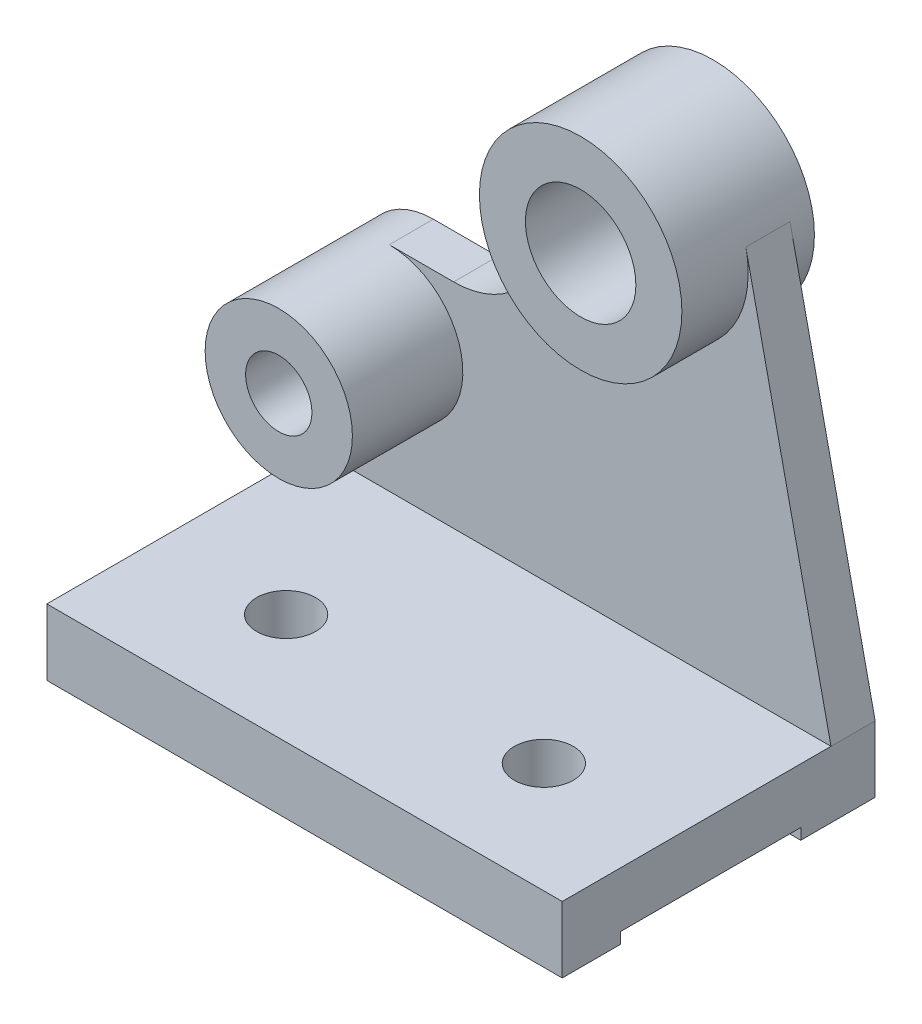
ISO-10303-21;
HEADER;
FILE_DESCRIPTION(('STEP AP214'),'2;1');
FILE_NAME('part.step','',(''),(''),'','','');
FILE_SCHEMA(('AUTOMOTIVE_DESIGN { 1 0 10303 214 1 1 1 1 }'));
ENDSEC;
DATA;
#1=APPLICATION_CONTEXT('core data for automotive mechanical design processes');
#2=APPLICATION_PROTOCOL_DEFINITION('international standard','automotive_design',2000,#1);
#3=PRODUCT_CONTEXT('',#1,'mechanical');
#4=PRODUCT('Part','Part','',(#3));
#5=PRODUCT_RELATED_PRODUCT_CATEGORY('part','',(#4));
#6=PRODUCT_DEFINITION_FORMATION('','',#4);
#7=PRODUCT_DEFINITION_CONTEXT('part definition',#1,'design');
#8=PRODUCT_DEFINITION('design','',#6,#7);
#9=PRODUCT_DEFINITION_SHAPE('','',#8);
#10=(LENGTH_UNIT() NAMED_UNIT(*) SI_UNIT(.MILLI.,.METRE.));
#11=(NAMED_UNIT(*) PLANE_ANGLE_UNIT() SI_UNIT($,.RADIAN.));
#12=(NAMED_UNIT(*) SI_UNIT($,.STERADIAN.) SOLID_ANGLE_UNIT());
#13=UNCERTAINTY_MEASURE_WITH_UNIT(LENGTH_MEASURE(1.E-05),#10,'distance_accuracy_value','');
#14=(GEOMETRIC_REPRESENTATION_CONTEXT(3) GLOBAL_UNCERTAINTY_ASSIGNED_CONTEXT((#13)) GLOBAL_UNIT_ASSIGNED_CONTEXT((#10,
#11,#12)) REPRESENTATION_CONTEXT('',''));
#15=CARTESIAN_POINT('',(0.,0.,0.));
#16=DIRECTION('',(0.,0.,1.));
#17=DIRECTION('',(1.,0.,0.));
#18=AXIS2_PLACEMENT_3D('',#15,#16,#17);
#19=CARTESIAN_POINT('',(-90.,-118.,85.));
#20=DIRECTION('',(0.,1.,0.));
#21=DIRECTION('',(0.,0.,1.));
#22=AXIS2_PLACEMENT_3D('',#19,#20,#21);
#23=PLANE('',#22);
#24=DIRECTION('',(0.,0.,-1.));
#25=VECTOR('',#24,1.);
#26=CARTESIAN_POINT('',(50.,-118.,85.));
#27=LINE('',#26,#25);
#28=CARTESIAN_POINT('',(50.0000000000001,-118.,20.2114764511151));
#29=VERTEX_POINT('',#28);
#30=CARTESIAN_POINT('',(50.,-118.,0.));
#31=VERTEX_POINT('',#30);
#32=EDGE_CURVE('E183',#29,#31,#27,.T.);
#33=ORIENTED_EDGE('',*,*,#32,.F.);
#34=DIRECTION('',(-1.,0.,0.));
#35=VECTOR('',#34,1.);
#36=CARTESIAN_POINT('',(50.0000000000001,-118.,20.2114764511151));
#37=LINE('',#36,#35);
#38=CARTESIAN_POINT('',(-90.,-118.,20.2114764511151));
#39=VERTEX_POINT('',#38);
#40=EDGE_CURVE('E240',#29,#39,#37,.T.);
#41=ORIENTED_EDGE('',*,*,#40,.T.);
#42=DIRECTION('',(0.,0.,-1.));
#43=VECTOR('',#42,1.);
#44=CARTESIAN_POINT('',(-90.,-118.,85.));
#45=LINE('',#44,#43);
#46=CARTESIAN_POINT('',(-90.,-118.,0.));
#47=VERTEX_POINT('',#46);
#48=EDGE_CURVE('E189',#39,#47,#45,.T.);
#49=ORIENTED_EDGE('',*,*,#48,.T.);
#50=DIRECTION('',(1.,0.,0.));
#51=VECTOR('',#50,1.);
#52=CARTESIAN_POINT('',(-90.,-118.,0.));
#53=LINE('',#52,#51);
#54=EDGE_CURVE('E279',#47,#31,#53,.T.);
#55=ORIENTED_EDGE('',*,*,#54,.T.);
#56=EDGE_LOOP('',(#33,#41,#49,#55));
#57=FACE_BOUND('',#56,.T.);
#58=ADVANCED_FACE('F41',(#57),#23,.F.);
#59=CARTESIAN_POINT('',(-70.,-62.,85.));
#60=DIRECTION('',(0.,0.,1.));
#61=DIRECTION('',(1.,0.,0.));
#62=AXIS2_PLACEMENT_3D('',#59,#60,#61);
#63=PLANE('',#62);
#64=DIRECTION('',(0.,1.,0.));
#65=VECTOR('',#64,1.);
#66=CARTESIAN_POINT('',(50.,-118.,85.));
#67=LINE('',#66,#65);
#68=CARTESIAN_POINT('',(50.,-118.,85.));
#69=VERTEX_POINT('',#68);
#70=CARTESIAN_POINT('',(50.,-100.,85.));
#71=VERTEX_POINT('',#70);
#72=EDGE_CURVE('E165',#69,#71,#67,.T.);
#73=ORIENTED_EDGE('',*,*,#72,.T.);
#74=DIRECTION('',(-1.,0.,0.));
#75=VECTOR('',#74,1.);
#76=CARTESIAN_POINT('',(50.,-100.,85.));
#77=LINE('',#76,#75);
#78=CARTESIAN_POINT('',(-90.,-100.,85.));
#79=VERTEX_POINT('',#78);
#80=EDGE_CURVE('E246',#71,#79,#77,.T.);
#81=ORIENTED_EDGE('',*,*,#80,.T.);
#82=DIRECTION('',(0.,-1.,0.));
#83=VECTOR('',#82,1.);
#84=CARTESIAN_POINT('',(-90.,-62.,85.));
#85=LINE('',#84,#83);
#86=CARTESIAN_POINT('',(-90.,-118.,85.));
#87=VERTEX_POINT('',#86);
#88=EDGE_CURVE('E272',#79,#87,#85,.T.);
#89=ORIENTED_EDGE('',*,*,#88,.T.);
#90=DIRECTION('',(1.,0.,0.));
#91=VECTOR('',#90,1.);
#92=CARTESIAN_POINT('',(-90.,-118.,85.));
#93=LINE('',#92,#91);
#94=EDGE_CURVE('E169',#87,#69,#93,.T.);
#95=ORIENTED_EDGE('',*,*,#94,.T.);
#96=EDGE_LOOP('',(#73,#81,#89,#95));
#97=FACE_BOUND('',#96,.T.);
#98=ADVANCED_FACE('F352',(#97),#63,.T.);
#99=CARTESIAN_POINT('',(-70.,-62.,85.));
#100=DIRECTION('',(0.,0.,-1.));
#101=DIRECTION('',(-1.,0.,0.));
#102=AXIS2_PLACEMENT_3D('',#99,#100,#101);
#103=CYLINDRICAL_SURFACE('',#102,20.);
#104=DIRECTION('',(0.,0.,-1.));
#105=VECTOR('',#104,1.);
#106=CARTESIAN_POINT('',(-90.,-62.,85.));
#107=LINE('',#106,#105);
#108=CARTESIAN_POINT('',(-90.,-62.,12.));
#109=VERTEX_POINT('',#108);
#110=CARTESIAN_POINT('',(-90.,-62.,0.));
#111=VERTEX_POINT('',#110);
#112=EDGE_CURVE('E151',#109,#111,#107,.T.);
#113=ORIENTED_EDGE('',*,*,#112,.F.);
#114=CARTESIAN_POINT('',(-70.,-62.,12.));
#115=DIRECTION('',(0.,0.,1.));
#116=DIRECTION('',(1.,0.,0.));
#117=AXIS2_PLACEMENT_3D('',#114,#115,#116);
#118=CIRCLE('',#117,20.);
#119=CARTESIAN_POINT('',(-70.,-42.,12.));
#120=VERTEX_POINT('',#119);
#121=EDGE_CURVE('E11',#120,#109,#118,.F.);
#122=ORIENTED_EDGE('',*,*,#121,.F.);
#123=DIRECTION('',(0.,0.,-1.));
#124=VECTOR('',#123,1.);
#125=CARTESIAN_POINT('',(-70.,-42.,85.));
#126=LINE('',#125,#124);
#127=CARTESIAN_POINT('',(-70.,-42.,0.));
#128=VERTEX_POINT('',#127);
#129=EDGE_CURVE('E146',#120,#128,#126,.T.);
#130=ORIENTED_EDGE('',*,*,#129,.T.);
#131=CARTESIAN_POINT('',(-70.,-62.,0.));
#132=DIRECTION('',(0.,0.,1.));
#133=DIRECTION('',(1.,0.,0.));
#134=AXIS2_PLACEMENT_3D('',#131,#132,#133);
#135=CIRCLE('',#134,20.);
#136=EDGE_CURVE('E269',#128,#111,#135,.T.);
#137=ORIENTED_EDGE('',*,*,#136,.T.);
#138=EDGE_LOOP('',(#113,#122,#130,#137));
#139=FACE_BOUND('',#138,.T.);
#140=CARTESIAN_POINT('',(-70.,-62.,42.));
#141=DIRECTION('',(0.,0.,1.));
#142=DIRECTION('',(1.,0.,0.));
#143=AXIS2_PLACEMENT_3D('',#140,#141,#142);
#144=CIRCLE('',#143,20.);
#145=CARTESIAN_POINT('',(-50.,-62.,42.));
#146=VERTEX_POINT('',#145);
#147=EDGE_CURVE('E208',#146,#146,#144,.T.);
#148=ORIENTED_EDGE('',*,*,#147,.F.);
#149=EDGE_LOOP('',(#148));
#150=FACE_BOUND('',#149,.T.);
#151=ADVANCED_FACE('F43',(#139,#150),#103,.T.);
#152=CARTESIAN_POINT('',(-90.,-62.,85.));
#153=DIRECTION('',(1.,0.,0.));
#154=DIRECTION('',(0.,1.,0.));
#155=AXIS2_PLACEMENT_3D('',#152,#153,#154);
#156=PLANE('',#155);
#157=ORIENTED_EDGE('',*,*,#48,.F.);
#158=DIRECTION('',(0.,-1.,0.));
#159=VECTOR('',#158,1.);
#160=CARTESIAN_POINT('',(-90.,-118.,20.2114764511151));
#161=LINE('',#160,#159);
#162=CARTESIAN_POINT('',(-90.,-115.,20.2114764511151));
#163=VERTEX_POINT('',#162);
#164=EDGE_CURVE('E226',#163,#39,#161,.T.);
#165=ORIENTED_EDGE('',*,*,#164,.F.);
#166=DIRECTION('',(0.,0.,-1.));
#167=VECTOR('',#166,1.);
#168=CARTESIAN_POINT('',(-90.,-115.,20.2114764511151));
#169=LINE('',#168,#167);
#170=CARTESIAN_POINT('',(-90.,-115.,69.2114764511151));
#171=VERTEX_POINT('',#170);
#172=EDGE_CURVE('E231',#171,#163,#169,.T.);
#173=ORIENTED_EDGE('',*,*,#172,.F.);
#174=DIRECTION('',(0.,1.,0.));
#175=VECTOR('',#174,1.);
#176=CARTESIAN_POINT('',(-90.,-118.,69.2114764511151));
#177=LINE('',#176,#175);
#178=CARTESIAN_POINT('',(-90.,-118.,69.2114764511151));
#179=VERTEX_POINT('',#178);
#180=EDGE_CURVE('E237',#179,#171,#177,.T.);
#181=ORIENTED_EDGE('',*,*,#180,.F.);
#182=EDGE_CURVE('E186',#87,#179,#45,.T.);
#183=ORIENTED_EDGE('',*,*,#182,.F.);
#184=ORIENTED_EDGE('',*,*,#88,.F.);
#185=DIRECTION('',(0.,0.,1.));
#186=VECTOR('',#185,1.);
#187=CARTESIAN_POINT('',(-90.,-100.,85.));
#188=LINE('',#187,#186);
#189=CARTESIAN_POINT('',(-90.,-100.,12.));
#190=VERTEX_POINT('',#189);
#191=EDGE_CURVE('E264',#190,#79,#188,.T.);
#192=ORIENTED_EDGE('',*,*,#191,.F.);
#193=DIRECTION('',(0.,-1.,0.));
#194=VECTOR('',#193,1.);
#195=CARTESIAN_POINT('',(-90.,-62.,12.));
#196=LINE('',#195,#194);
#197=EDGE_CURVE('E263',#109,#190,#196,.T.);
#198=ORIENTED_EDGE('',*,*,#197,.F.);
#199=ORIENTED_EDGE('',*,*,#112,.T.);
#200=DIRECTION('',(0.,-1.,0.));
#201=VECTOR('',#200,1.);
#202=CARTESIAN_POINT('',(-90.,-62.,0.));
#203=LINE('',#202,#201);
#204=EDGE_CURVE('E273',#111,#47,#203,.T.);
#205=ORIENTED_EDGE('',*,*,#204,.T.);
#206=EDGE_LOOP('',(#157,#165,#173,#181,#183,#184,#192,#198,#199,#205));
#207=FACE_BOUND('',#206,.T.);
#208=ADVANCED_FACE('F303',(#207),#156,.F.);
#209=CARTESIAN_POINT('',(50.,-100.,85.));
#210=DIRECTION('',(-0.97694867206773,-0.213474336033865,0.));
#211=DIRECTION('',(0.213474336033865,-0.97694867206773,0.));
#212=AXIS2_PLACEMENT_3D('',#209,#210,#211);
#213=PLANE('',#212);
#214=DIRECTION('',(-0.213474336033865,0.97694867206773,0.));
#215=VECTOR('',#214,1.);
#216=CARTESIAN_POINT('',(50.,-100.,12.));
#217=LINE('',#216,#215);
#218=CARTESIAN_POINT('',(50.,-100.,12.));
#219=VERTEX_POINT('',#218);
#220=CARTESIAN_POINT('',(26.8660884818626,5.87054424093129,12.));
#221=VERTEX_POINT('',#220);
#222=EDGE_CURVE('E258',#219,#221,#217,.T.);
#223=ORIENTED_EDGE('',*,*,#222,.F.);
#224=DIRECTION('',(0.,0.,-1.));
#225=VECTOR('',#224,1.);
#226=CARTESIAN_POINT('',(50.,-100.,85.));
#227=LINE('',#226,#225);
#228=CARTESIAN_POINT('',(50.,-100.,0.));
#229=VERTEX_POINT('',#228);
#230=EDGE_CURVE('E181',#219,#229,#227,.T.);
#231=ORIENTED_EDGE('',*,*,#230,.T.);
#232=DIRECTION('',(-0.213474336033865,0.97694867206773,0.));
#233=VECTOR('',#232,1.);
#234=CARTESIAN_POINT('',(50.,-100.,0.));
#235=LINE('',#234,#233);
#236=CARTESIAN_POINT('',(26.8660884818626,5.87054424093128,0.));
#237=VERTEX_POINT('',#236);
#238=EDGE_CURVE('E282',#229,#237,#235,.T.);
#239=ORIENTED_EDGE('',*,*,#238,.T.);
#240=DIRECTION('',(0.,0.,-1.));
#241=VECTOR('',#240,1.);
#242=CARTESIAN_POINT('',(26.8660884818626,5.87054424093128,85.));
#243=LINE('',#242,#241);
#244=EDGE_CURVE('E178',#221,#237,#243,.T.);
#245=ORIENTED_EDGE('',*,*,#244,.F.);
#246=EDGE_LOOP('',(#223,#231,#239,#245));
#247=FACE_BOUND('',#246,.T.);
#248=ADVANCED_FACE('F319',(#247),#213,.F.);
#249=CARTESIAN_POINT('',(0.,0.,85.));
#250=DIRECTION('',(0.,0.,-1.));
#251=DIRECTION('',(-1.,0.,0.));
#252=AXIS2_PLACEMENT_3D('',#249,#250,#251);
#253=CYLINDRICAL_SURFACE('',#252,27.5);
#254=DIRECTION('',(0.,0.,-1.));
#255=VECTOR('',#254,1.);
#256=CARTESIAN_POINT('',(-27.5,0.,85.));
#257=LINE('',#256,#255);
#258=CARTESIAN_POINT('',(-27.5,0.,12.));
#259=VERTEX_POINT('',#258);
#260=CARTESIAN_POINT('',(-27.5,0.,0.));
#261=VERTEX_POINT('',#260);
#262=EDGE_CURVE('E174',#259,#261,#257,.T.);
#263=ORIENTED_EDGE('',*,*,#262,.F.);
#264=CARTESIAN_POINT('',(0.,0.,12.));
#265=DIRECTION('',(0.,0.,1.));
#266=DIRECTION('',(1.,0.,0.));
#267=AXIS2_PLACEMENT_3D('',#264,#265,#266);
#268=CIRCLE('',#267,27.5);
#269=EDGE_CURVE('E49',#221,#259,#268,.F.);
#270=ORIENTED_EDGE('',*,*,#269,.F.);
#271=ORIENTED_EDGE('',*,*,#244,.T.);
#272=CARTESIAN_POINT('',(0.,0.,0.));
#273=DIRECTION('',(0.,0.,1.));
#274=DIRECTION('',(1.,0.,0.));
#275=AXIS2_PLACEMENT_3D('',#272,#273,#274);
#276=CIRCLE('',#275,27.5);
#277=EDGE_CURVE('E221',#237,#261,#276,.F.);
#278=ORIENTED_EDGE('',*,*,#277,.T.);
#279=EDGE_LOOP('',(#263,#270,#271,#278));
#280=FACE_BOUND('',#279,.T.);
#281=CARTESIAN_POINT('',(0.,0.,30.));
#282=DIRECTION('',(0.,0.,1.));
#283=DIRECTION('',(1.,0.,0.));
#284=AXIS2_PLACEMENT_3D('',#281,#282,#283);
#285=CIRCLE('',#284,27.5);
#286=CARTESIAN_POINT('',(27.5,0.,30.));
#287=VERTEX_POINT('',#286);
#288=EDGE_CURVE('E220',#287,#287,#285,.T.);
#289=ORIENTED_EDGE('',*,*,#288,.F.);
#290=EDGE_LOOP('',(#289));
#291=FACE_BOUND('',#290,.T.);
#292=CARTESIAN_POINT('',(0.,0.,-5.99999999999999));
#293=DIRECTION('',(0.,0.,1.));
#294=DIRECTION('',(1.,0.,0.));
#295=AXIS2_PLACEMENT_3D('',#292,#293,#294);
#296=CIRCLE('',#295,27.5);
#297=CARTESIAN_POINT('',(27.5,0.,-5.99999999999999));
#298=VERTEX_POINT('',#297);
#299=EDGE_CURVE('E218',#298,#298,#296,.T.);
#300=ORIENTED_EDGE('',*,*,#299,.T.);
#301=EDGE_LOOP('',(#300));
#302=FACE_BOUND('',#301,.T.);
#303=ADVANCED_FACE('F323',(#280,#291,#302),#253,.T.);
#304=CARTESIAN_POINT('',(-27.5,0.,85.));
#305=DIRECTION('',(1.,0.,0.));
#306=DIRECTION('',(0.,0.,-1.));
#307=AXIS2_PLACEMENT_3D('',#304,#305,#306);
#308=PLANE('',#307);
#309=DIRECTION('',(0.,-1.,0.));
#310=VECTOR('',#309,1.);
#311=CARTESIAN_POINT('',(-27.5,0.,12.));
#312=LINE('',#311,#310);
#313=CARTESIAN_POINT('',(-27.5,-17.,12.));
#314=VERTEX_POINT('',#313);
#315=EDGE_CURVE('E259',#259,#314,#312,.T.);
#316=ORIENTED_EDGE('',*,*,#315,.F.);
#317=ORIENTED_EDGE('',*,*,#262,.T.);
#318=DIRECTION('',(0.,-1.,0.));
#319=VECTOR('',#318,1.);
#320=CARTESIAN_POINT('',(-27.5,0.,0.));
#321=LINE('',#320,#319);
#322=CARTESIAN_POINT('',(-27.5,-16.9999999999998,0.));
#323=VERTEX_POINT('',#322);
#324=EDGE_CURVE('E290',#261,#323,#321,.T.);
#325=ORIENTED_EDGE('',*,*,#324,.T.);
#326=DIRECTION('',(0.,0.,-1.));
#327=VECTOR('',#326,1.);
#328=CARTESIAN_POINT('',(-27.5,-16.9999999999998,85.));
#329=LINE('',#328,#327);
#330=EDGE_CURVE('E168',#314,#323,#329,.T.);
#331=ORIENTED_EDGE('',*,*,#330,.F.);
#332=EDGE_LOOP('',(#316,#317,#325,#331));
#333=FACE_BOUND('',#332,.T.);
#334=ADVANCED_FACE('F321',(#333),#308,.F.);
#335=CARTESIAN_POINT('',(-52.5,-17.,85.));
#336=DIRECTION('',(0.,0.,-1.));
#337=DIRECTION('',(-1.,0.,0.));
#338=AXIS2_PLACEMENT_3D('',#335,#336,#337);
#339=CYLINDRICAL_SURFACE('',#338,25.);
#340=CARTESIAN_POINT('',(-52.5,-17.,12.));
#341=DIRECTION('',(0.,0.,1.));
#342=DIRECTION('',(1.,0.,0.));
#343=AXIS2_PLACEMENT_3D('',#340,#341,#342);
#344=CIRCLE('',#343,25.);
#345=CARTESIAN_POINT('',(-52.5000000000002,-42.,12.));
#346=VERTEX_POINT('',#345);
#347=EDGE_CURVE('E66',#314,#346,#344,.F.);
#348=ORIENTED_EDGE('',*,*,#347,.F.);
#349=ORIENTED_EDGE('',*,*,#330,.T.);
#350=CARTESIAN_POINT('',(-52.5,-17.,0.));
#351=DIRECTION('',(0.,0.,-1.));
#352=DIRECTION('',(-1.,0.,0.));
#353=AXIS2_PLACEMENT_3D('',#350,#351,#352);
#354=CIRCLE('',#353,25.);
#355=CARTESIAN_POINT('',(-52.5000000000002,-42.,0.));
#356=VERTEX_POINT('',#355);
#357=EDGE_CURVE('E287',#323,#356,#354,.T.);
#358=ORIENTED_EDGE('',*,*,#357,.T.);
#359=DIRECTION('',(0.,0.,-1.));
#360=VECTOR('',#359,1.);
#361=CARTESIAN_POINT('',(-52.5000000000002,-42.,85.));
#362=LINE('',#361,#360);
#363=EDGE_CURVE('E161',#346,#356,#362,.T.);
#364=ORIENTED_EDGE('',*,*,#363,.F.);
#365=EDGE_LOOP('',(#348,#349,#358,#364));
#366=FACE_BOUND('',#365,.T.);
#367=ADVANCED_FACE('F291',(#366),#339,.F.);
#368=CARTESIAN_POINT('',(-52.5000000000002,-42.,85.));
#369=DIRECTION('',(0.,-1.,0.));
#370=DIRECTION('',(0.,0.,-1.));
#371=AXIS2_PLACEMENT_3D('',#368,#369,#370);
#372=PLANE('',#371);
#373=DIRECTION('',(-1.,0.,0.));
#374=VECTOR('',#373,1.);
#375=CARTESIAN_POINT('',(-52.5000000000002,-42.,12.));
#376=LINE('',#375,#374);
#377=EDGE_CURVE('E153',#346,#120,#376,.T.);
#378=ORIENTED_EDGE('',*,*,#377,.F.);
#379=ORIENTED_EDGE('',*,*,#363,.T.);
#380=DIRECTION('',(-1.,0.,0.));
#381=VECTOR('',#380,1.);
#382=CARTESIAN_POINT('',(-52.5000000000002,-42.,0.));
#383=LINE('',#382,#381);
#384=EDGE_CURVE('E163',#356,#128,#383,.T.);
#385=ORIENTED_EDGE('',*,*,#384,.T.);
#386=ORIENTED_EDGE('',*,*,#129,.F.);
#387=EDGE_LOOP('',(#378,#379,#385,#386));
#388=FACE_BOUND('',#387,.T.);
#389=ADVANCED_FACE('F157',(#388),#372,.F.);
#390=CARTESIAN_POINT('',(-70.,-62.,85.));
#391=DIRECTION('',(0.,0.,-1.));
#392=DIRECTION('',(-1.,0.,0.));
#393=AXIS2_PLACEMENT_3D('',#390,#391,#392);
#394=CYLINDRICAL_SURFACE('',#393,9.);
#395=CARTESIAN_POINT('',(-70.,-62.,0.));
#396=DIRECTION('',(0.,0.,1.));
#397=DIRECTION('',(1.,0.,0.));
#398=AXIS2_PLACEMENT_3D('',#395,#396,#397);
#399=CIRCLE('',#398,9.);
#400=CARTESIAN_POINT('',(-61.,-62.,0.));
#401=VERTEX_POINT('',#400);
#402=EDGE_CURVE('E270',#401,#401,#399,.T.);
#403=ORIENTED_EDGE('',*,*,#402,.F.);
#404=EDGE_LOOP('',(#403));
#405=FACE_BOUND('',#404,.T.);
#406=CARTESIAN_POINT('',(-70.,-62.,42.));
#407=DIRECTION('',(0.,0.,1.));
#408=DIRECTION('',(1.,0.,0.));
#409=AXIS2_PLACEMENT_3D('',#406,#407,#408);
#410=CIRCLE('',#409,9.);
#411=CARTESIAN_POINT('',(-61.,-62.,42.));
#412=VERTEX_POINT('',#411);
#413=EDGE_CURVE('E197',#412,#412,#410,.F.);
#414=ORIENTED_EDGE('',*,*,#413,.F.);
#415=EDGE_LOOP('',(#414));
#416=FACE_BOUND('',#415,.T.);
#417=ADVANCED_FACE('F375',(#405,#416),#394,.F.);
#418=CARTESIAN_POINT('',(-70.,-62.,0.));
#419=DIRECTION('',(0.,0.,1.));
#420=DIRECTION('',(1.,0.,0.));
#421=AXIS2_PLACEMENT_3D('',#418,#419,#420);
#422=PLANE('',#421);
#423=ORIENTED_EDGE('',*,*,#277,.F.);
#424=ORIENTED_EDGE('',*,*,#238,.F.);
#425=DIRECTION('',(0.,1.,0.));
#426=VECTOR('',#425,1.);
#427=CARTESIAN_POINT('',(50.,-118.,0.));
#428=LINE('',#427,#426);
#429=EDGE_CURVE('E281',#31,#229,#428,.T.);
#430=ORIENTED_EDGE('',*,*,#429,.F.);
#431=ORIENTED_EDGE('',*,*,#54,.F.);
#432=ORIENTED_EDGE('',*,*,#204,.F.);
#433=ORIENTED_EDGE('',*,*,#136,.F.);
#434=ORIENTED_EDGE('',*,*,#384,.F.);
#435=ORIENTED_EDGE('',*,*,#357,.F.);
#436=ORIENTED_EDGE('',*,*,#324,.F.);
#437=EDGE_LOOP('',(#423,#424,#430,#431,#432,#433,#434,#435,#436));
#438=FACE_BOUND('',#437,.T.);
#439=ORIENTED_EDGE('',*,*,#402,.T.);
#440=EDGE_LOOP('',(#439));
#441=FACE_BOUND('',#440,.T.);
#442=ADVANCED_FACE('F298',(#438,#441),#422,.F.);
#443=ORIENTED_EDGE('',*,*,#182,.T.);
#444=DIRECTION('',(-1.,0.,0.));
#445=VECTOR('',#444,1.);
#446=CARTESIAN_POINT('',(50.0000000000001,-118.,69.2114764511151));
#447=LINE('',#446,#445);
#448=CARTESIAN_POINT('',(50.0000000000001,-118.,69.2114764511151));
#449=VERTEX_POINT('',#448);
#450=EDGE_CURVE('E248',#449,#179,#447,.T.);
#451=ORIENTED_EDGE('',*,*,#450,.F.);
#452=EDGE_CURVE('E184',#69,#449,#27,.T.);
#453=ORIENTED_EDGE('',*,*,#452,.F.);
#454=ORIENTED_EDGE('',*,*,#94,.F.);
#455=EDGE_LOOP('',(#443,#451,#453,#454));
#456=FACE_BOUND('',#455,.T.);
#457=ADVANCED_FACE('F357',(#456),#23,.F.);
#458=CARTESIAN_POINT('',(50.,-118.,85.));
#459=DIRECTION('',(-1.,0.,0.));
#460=DIRECTION('',(0.,-1.,0.));
#461=AXIS2_PLACEMENT_3D('',#458,#459,#460);
#462=PLANE('',#461);
#463=DIRECTION('',(0.,0.,-1.));
#464=VECTOR('',#463,1.);
#465=CARTESIAN_POINT('',(50.0000000000001,-115.,20.2114764511151));
#466=LINE('',#465,#464);
#467=CARTESIAN_POINT('',(50.,-115.,69.2114764511151));
#468=VERTEX_POINT('',#467);
#469=CARTESIAN_POINT('',(50.0000000000001,-115.,20.2114764511151));
#470=VERTEX_POINT('',#469);
#471=EDGE_CURVE('E59',#468,#470,#466,.T.);
#472=ORIENTED_EDGE('',*,*,#471,.T.);
#473=DIRECTION('',(0.,-1.,0.));
#474=VECTOR('',#473,1.);
#475=CARTESIAN_POINT('',(50.0000000000001,-118.,20.2114764511151));
#476=LINE('',#475,#474);
#477=EDGE_CURVE('E230',#470,#29,#476,.T.);
#478=ORIENTED_EDGE('',*,*,#477,.T.);
#479=ORIENTED_EDGE('',*,*,#32,.T.);
#480=ORIENTED_EDGE('',*,*,#429,.T.);
#481=ORIENTED_EDGE('',*,*,#230,.F.);
#482=EDGE_CURVE('E185',#71,#219,#227,.T.);
#483=ORIENTED_EDGE('',*,*,#482,.F.);
#484=ORIENTED_EDGE('',*,*,#72,.F.);
#485=ORIENTED_EDGE('',*,*,#452,.T.);
#486=DIRECTION('',(0.,1.,0.));
#487=VECTOR('',#486,1.);
#488=CARTESIAN_POINT('',(50.0000000000001,-118.,69.2114764511151));
#489=LINE('',#488,#487);
#490=EDGE_CURVE('E235',#449,#468,#489,.T.);
#491=ORIENTED_EDGE('',*,*,#490,.T.);
#492=EDGE_LOOP('',(#472,#478,#479,#480,#481,#483,#484,#485,#491));
#493=FACE_BOUND('',#492,.T.);
#494=ADVANCED_FACE('F314',(#493),#462,.F.);
#495=CARTESIAN_POINT('',(50.,-100.,12.));
#496=DIRECTION('',(0.,1.,0.));
#497=DIRECTION('',(-1.,0.,0.));
#498=AXIS2_PLACEMENT_3D('',#495,#496,#497);
#499=PLANE('',#498);
#500=CARTESIAN_POINT('',(-55.,-100.,55.));
#501=DIRECTION('',(0.,1.,0.));
#502=DIRECTION('',(-1.,0.,0.));
#503=AXIS2_PLACEMENT_3D('',#500,#501,#502);
#504=CIRCLE('',#503,8.);
#505=CARTESIAN_POINT('',(-63.,-100.,55.));
#506=VERTEX_POINT('',#505);
#507=EDGE_CURVE('E193',#506,#506,#504,.T.);
#508=ORIENTED_EDGE('',*,*,#507,.F.);
#509=EDGE_LOOP('',(#508));
#510=FACE_BOUND('',#509,.T.);
#511=CARTESIAN_POINT('',(15.,-100.,55.));
#512=DIRECTION('',(0.,1.,0.));
#513=DIRECTION('',(-1.,0.,0.));
#514=AXIS2_PLACEMENT_3D('',#511,#512,#513);
#515=CIRCLE('',#514,8.);
#516=CARTESIAN_POINT('',(7.,-100.,55.));
#517=VERTEX_POINT('',#516);
#518=EDGE_CURVE('E201',#517,#517,#515,.T.);
#519=ORIENTED_EDGE('',*,*,#518,.F.);
#520=EDGE_LOOP('',(#519));
#521=FACE_BOUND('',#520,.T.);
#522=ORIENTED_EDGE('',*,*,#191,.T.);
#523=ORIENTED_EDGE('',*,*,#80,.F.);
#524=ORIENTED_EDGE('',*,*,#482,.T.);
#525=DIRECTION('',(-1.,0.,0.));
#526=VECTOR('',#525,1.);
#527=CARTESIAN_POINT('',(50.,-100.,12.));
#528=LINE('',#527,#526);
#529=EDGE_CURVE('E160',#219,#190,#528,.T.);
#530=ORIENTED_EDGE('',*,*,#529,.T.);
#531=EDGE_LOOP('',(#522,#523,#524,#530));
#532=FACE_BOUND('',#531,.T.);
#533=ADVANCED_FACE('F309',(#510,#521,#532),#499,.T.);
#534=CARTESIAN_POINT('',(0.,0.,12.));
#535=DIRECTION('',(0.,0.,1.));
#536=DIRECTION('',(1.,0.,0.));
#537=AXIS2_PLACEMENT_3D('',#534,#535,#536);
#538=PLANE('',#537);
#539=ORIENTED_EDGE('',*,*,#377,.T.);
#540=ORIENTED_EDGE('',*,*,#121,.T.);
#541=ORIENTED_EDGE('',*,*,#197,.T.);
#542=ORIENTED_EDGE('',*,*,#529,.F.);
#543=ORIENTED_EDGE('',*,*,#222,.T.);
#544=ORIENTED_EDGE('',*,*,#269,.T.);
#545=ORIENTED_EDGE('',*,*,#315,.T.);
#546=ORIENTED_EDGE('',*,*,#347,.T.);
#547=EDGE_LOOP('',(#539,#540,#541,#542,#543,#544,#545,#546));
#548=FACE_BOUND('',#547,.T.);
#549=ADVANCED_FACE('F152',(#548),#538,.T.);
#550=CARTESIAN_POINT('',(50.0000000000001,-118.,20.2114764511151));
#551=DIRECTION('',(0.,0.,-1.));
#552=DIRECTION('',(-1.,0.,0.));
#553=AXIS2_PLACEMENT_3D('',#550,#551,#552);
#554=PLANE('',#553);
#555=ORIENTED_EDGE('',*,*,#164,.T.);
#556=ORIENTED_EDGE('',*,*,#40,.F.);
#557=ORIENTED_EDGE('',*,*,#477,.F.);
#558=DIRECTION('',(-1.,0.,0.));
#559=VECTOR('',#558,1.);
#560=CARTESIAN_POINT('',(50.0000000000001,-115.,20.2114764511151));
#561=LINE('',#560,#559);
#562=EDGE_CURVE('E242',#470,#163,#561,.T.);
#563=ORIENTED_EDGE('',*,*,#562,.T.);
#564=EDGE_LOOP('',(#555,#556,#557,#563));
#565=FACE_BOUND('',#564,.T.);
#566=ADVANCED_FACE('F381',(#565),#554,.F.);
#567=CARTESIAN_POINT('',(50.0000000000001,-115.,20.2114764511151));
#568=DIRECTION('',(0.,1.,0.));
#569=DIRECTION('',(-1.,0.,0.));
#570=AXIS2_PLACEMENT_3D('',#567,#568,#569);
#571=PLANE('',#570);
#572=CARTESIAN_POINT('',(-55.,-115.,55.));
#573=DIRECTION('',(0.,1.,0.));
#574=DIRECTION('',(-1.,0.,0.));
#575=AXIS2_PLACEMENT_3D('',#572,#573,#574);
#576=CIRCLE('',#575,8.);
#577=CARTESIAN_POINT('',(-63.,-115.,55.));
#578=VERTEX_POINT('',#577);
#579=EDGE_CURVE('E44',#578,#578,#576,.T.);
#580=ORIENTED_EDGE('',*,*,#579,.T.);
#581=EDGE_LOOP('',(#580));
#582=FACE_BOUND('',#581,.T.);
#583=CARTESIAN_POINT('',(15.,-115.,55.));
#584=DIRECTION('',(0.,1.,0.));
#585=DIRECTION('',(-1.,0.,0.));
#586=AXIS2_PLACEMENT_3D('',#583,#584,#585);
#587=CIRCLE('',#586,8.);
#588=CARTESIAN_POINT('',(7.,-115.,55.));
#589=VERTEX_POINT('',#588);
#590=EDGE_CURVE('E194',#589,#589,#587,.T.);
#591=ORIENTED_EDGE('',*,*,#590,.T.);
#592=EDGE_LOOP('',(#591));
#593=FACE_BOUND('',#592,.T.);
#594=ORIENTED_EDGE('',*,*,#172,.T.);
#595=ORIENTED_EDGE('',*,*,#562,.F.);
#596=ORIENTED_EDGE('',*,*,#471,.F.);
#597=DIRECTION('',(-1.,0.,0.));
#598=VECTOR('',#597,1.);
#599=CARTESIAN_POINT('',(50.0000000000001,-115.,69.2114764511151));
#600=LINE('',#599,#598);
#601=EDGE_CURVE('E250',#468,#171,#600,.T.);
#602=ORIENTED_EDGE('',*,*,#601,.T.);
#603=EDGE_LOOP('',(#594,#595,#596,#602));
#604=FACE_BOUND('',#603,.T.);
#605=ADVANCED_FACE('F383',(#582,#593,#604),#571,.F.);
#606=CARTESIAN_POINT('',(50.0000000000001,-118.,69.2114764511151));
#607=DIRECTION('',(0.,0.,1.));
#608=DIRECTION('',(1.,0.,0.));
#609=AXIS2_PLACEMENT_3D('',#606,#607,#608);
#610=PLANE('',#609);
#611=ORIENTED_EDGE('',*,*,#180,.T.);
#612=ORIENTED_EDGE('',*,*,#601,.F.);
#613=ORIENTED_EDGE('',*,*,#490,.F.);
#614=ORIENTED_EDGE('',*,*,#450,.T.);
#615=EDGE_LOOP('',(#611,#612,#613,#614));
#616=FACE_BOUND('',#615,.T.);
#617=ADVANCED_FACE('F382',(#616),#610,.F.);
#618=CARTESIAN_POINT('',(0.,0.,30.));
#619=DIRECTION('',(0.,0.,1.));
#620=DIRECTION('',(1.,0.,0.));
#621=AXIS2_PLACEMENT_3D('',#618,#619,#620);
#622=PLANE('',#621);
#623=CARTESIAN_POINT('',(0.,0.,30.));
#624=DIRECTION('',(0.,0.,1.));
#625=DIRECTION('',(1.,0.,0.));
#626=AXIS2_PLACEMENT_3D('',#623,#624,#625);
#627=CIRCLE('',#626,15.);
#628=CARTESIAN_POINT('',(15.,0.,30.));
#629=VERTEX_POINT('',#628);
#630=EDGE_CURVE('E211',#629,#629,#627,.F.);
#631=ORIENTED_EDGE('',*,*,#630,.T.);
#632=EDGE_LOOP('',(#631));
#633=FACE_BOUND('',#632,.T.);
#634=ORIENTED_EDGE('',*,*,#288,.T.);
#635=EDGE_LOOP('',(#634));
#636=FACE_BOUND('',#635,.T.);
#637=ADVANCED_FACE('F350',(#633,#636),#622,.T.);
#638=CARTESIAN_POINT('',(0.,0.,85.));
#639=DIRECTION('',(0.,0.,-1.));
#640=DIRECTION('',(-1.,0.,0.));
#641=AXIS2_PLACEMENT_3D('',#638,#639,#640);
#642=CYLINDRICAL_SURFACE('',#641,15.);
#643=ORIENTED_EDGE('',*,*,#630,.F.);
#644=EDGE_LOOP('',(#643));
#645=FACE_BOUND('',#644,.T.);
#646=CARTESIAN_POINT('',(0.,0.,-5.99999999999999));
#647=DIRECTION('',(0.,0.,1.));
#648=DIRECTION('',(1.,0.,0.));
#649=AXIS2_PLACEMENT_3D('',#646,#647,#648);
#650=CIRCLE('',#649,15.);
#651=CARTESIAN_POINT('',(15.,0.,-5.99999999999999));
#652=VERTEX_POINT('',#651);
#653=EDGE_CURVE('E214',#652,#652,#650,.F.);
#654=ORIENTED_EDGE('',*,*,#653,.T.);
#655=EDGE_LOOP('',(#654));
#656=FACE_BOUND('',#655,.T.);
#657=ADVANCED_FACE('F337',(#645,#656),#642,.F.);
#658=CARTESIAN_POINT('',(0.,0.,-5.99999999999999));
#659=DIRECTION('',(0.,0.,1.));
#660=DIRECTION('',(1.,0.,0.));
#661=AXIS2_PLACEMENT_3D('',#658,#659,#660);
#662=PLANE('',#661);
#663=ORIENTED_EDGE('',*,*,#653,.F.);
#664=EDGE_LOOP('',(#663));
#665=FACE_BOUND('',#664,.T.);
#666=ORIENTED_EDGE('',*,*,#299,.F.);
#667=EDGE_LOOP('',(#666));
#668=FACE_BOUND('',#667,.T.);
#669=ADVANCED_FACE('F333',(#665,#668),#662,.F.);
#670=CARTESIAN_POINT('',(0.,0.,42.));
#671=DIRECTION('',(0.,0.,1.));
#672=DIRECTION('',(1.,0.,0.));
#673=AXIS2_PLACEMENT_3D('',#670,#671,#672);
#674=PLANE('',#673);
#675=ORIENTED_EDGE('',*,*,#413,.T.);
#676=EDGE_LOOP('',(#675));
#677=FACE_BOUND('',#676,.T.);
#678=ORIENTED_EDGE('',*,*,#147,.T.);
#679=EDGE_LOOP('',(#678));
#680=FACE_BOUND('',#679,.T.);
#681=ADVANCED_FACE('F334',(#677,#680),#674,.T.);
#682=CARTESIAN_POINT('',(15.,-130.,55.));
#683=DIRECTION('',(0.,1.,0.));
#684=DIRECTION('',(-1.,0.,0.));
#685=AXIS2_PLACEMENT_3D('',#682,#683,#684);
#686=CYLINDRICAL_SURFACE('',#685,8.);
#687=ORIENTED_EDGE('',*,*,#518,.T.);
#688=EDGE_LOOP('',(#687));
#689=FACE_BOUND('',#688,.T.);
#690=ORIENTED_EDGE('',*,*,#590,.F.);
#691=EDGE_LOOP('',(#690));
#692=FACE_BOUND('',#691,.T.);
#693=ADVANCED_FACE('F341',(#689,#692),#686,.F.);
#694=CARTESIAN_POINT('',(-55.,-130.,55.));
#695=DIRECTION('',(0.,1.,0.));
#696=DIRECTION('',(-1.,0.,0.));
#697=AXIS2_PLACEMENT_3D('',#694,#695,#696);
#698=CYLINDRICAL_SURFACE('',#697,8.);
#699=ORIENTED_EDGE('',*,*,#507,.T.);
#700=EDGE_LOOP('',(#699));
#701=FACE_BOUND('',#700,.T.);
#702=ORIENTED_EDGE('',*,*,#579,.F.);
#703=EDGE_LOOP('',(#702));
#704=FACE_BOUND('',#703,.T.);
#705=ADVANCED_FACE('F450',(#701,#704),#698,.F.);
#706=CLOSED_SHELL('',(#58,#98,#151,#208,#248,#303,#334,#367,#389,#417,#442,#457,#494,#533,#549,
#566,#605,#617,#637,#657,#669,#681,#693,#705));
#707=MANIFOLD_SOLID_BREP('B2',#706);
#708=ADVANCED_BREP_SHAPE_REPRESENTATION('',(#18,#707),#14);
#709=SHAPE_DEFINITION_REPRESENTATION(#9,#708);
ENDSEC;
END-ISO-10303-21;
